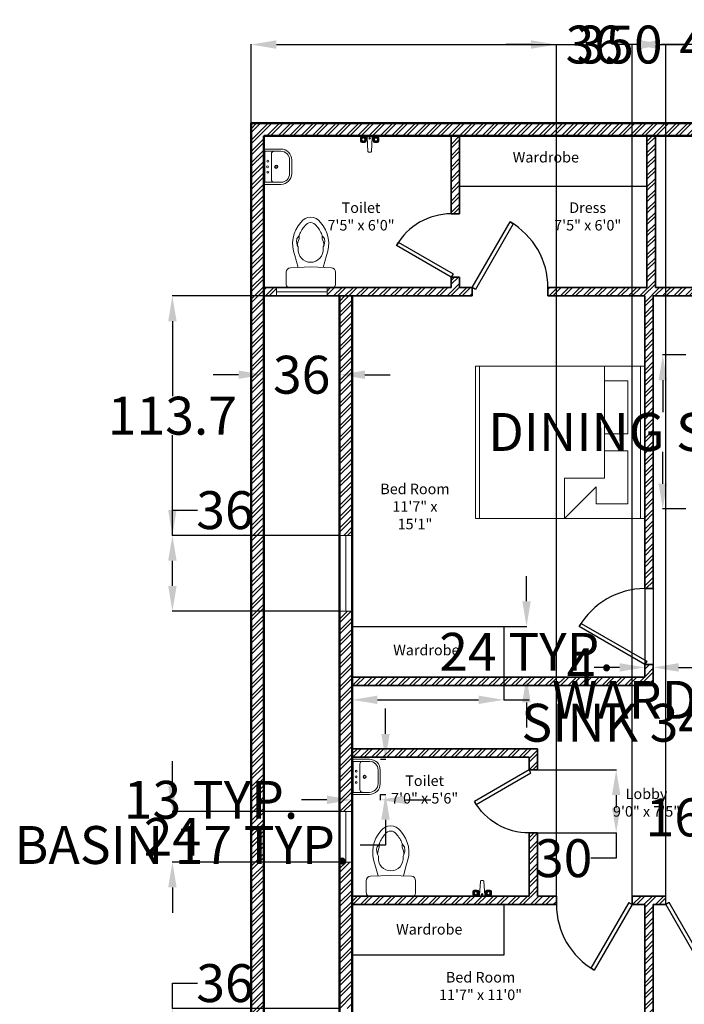
# Model space of a CAD drawing. Units: inches. Extents: x 73 to 1216, y -495 to 328.
# Tile 2 of 9: x 73 to 389, y -139 to 328. Entities that reach past the tile are written whole.
import ezdxf

# ---------------------------------------------------------------- set-up
doc = ezdxf.new("R2010")
doc.units = ezdxf.units.IN
for name, color, linetype, lineweight in [('A-ANNO-DIMS', 2, 'Continuous', 18), ('A-AREA-IDEN', 7, 'Continuous', 18), ('A-DOOR', 3, 'Continuous', 25), ('A-FLOR-CASE', 2, 'Continuous', 25), ('A-FLOR-FIXT', 9, 'Continuous', 18), ('A-GLAZ', 3, 'Continuous', 18), ('A-WALL-PATT', 8, 'Continuous', 13), ('Furniture', 2, 'Continuous', 18), ('Inner Walls', 5, 'Continuous', 35), ('Outer Walls', 1, 'Continuous', 50), ('Text-T18', 7, 'Continuous', 18)]:
    doc.layers.add(name, color=color, linetype=linetype, lineweight=lineweight)
doc.styles.get("Standard").update_dxf_attribs({"font": 'arial.ttf'})
doc.dimstyles.get("Standard").update_dxf_attribs({"dimtxt": 18, "dimasz": 12, "dimexe": 0.18, "dimexo": 0.0625, "dimgap": 0.09, "dimtad": 0, "dimtih": 1, "dimtoh": 1, "dimdec": 0, "dimzin": 0, "dimdsep": 46, "dimlunit": 3, "dimtxsty": 'Standard', "dimcen": 0.09, "dimadec": 0, "dimazin": 0, "dimtfac": 1, "dimtdec": 0, "dimtofl": 0, "dimtmove": 0, "dimatfit": 3, "dimfxl": 1, "dimtolj": 1, "dimtzin": 0, "dimarcsym": 0})
pattern_1 = [(45, (-434.707, -1257.0093), (-2.694077, 2.694077), []), (45, (-432.911, -1257.0093), (-2.694077, 2.694077), [])]

# ---------------------------------------------------------------- blocks, each defined once
blk = doc.blocks.new('*U2')
for p, q in [((0, 0), (0, -4)), ((36, 0), (36, -4))]:
    blk.add_line(p, q)
blk.add_lwpolyline([(0, 0), (18, 31.18), (19.52, 30.3), (1.52, -0.88)], close=True)
blk.add_arc((0, 0), 36, 0, 60)
blk = doc.blocks.new('*U3')
for p, q in [((0, 0), (0, -4)), ((30, 0), (30, -4))]:
    blk.add_line(p, q)
blk.add_lwpolyline([(0, 0), (15, 25.98), (16.52, 25.11), (1.52, -0.88)], close=True)
blk.add_arc((0, 0), 30, 0, 60)
blk = doc.blocks.new('*U4')
for p, q in [((0, 0), (0, -4)), ((40, 0), (40, -4))]:
    blk.add_line(p, q)
blk.add_lwpolyline([(0, 0), (20, 34.64), (21.52, 33.77), (1.52, -0.88)], close=True)
blk.add_arc((0, 0), 40, 0, 60)
blk = doc.blocks.new('KING-00')
for p, q in [((-0.897, -0.947), (-0.897, 0.882)), ((0.602, 0.882), (0.602, -0.464)), ((1.034, -0.947), (1.034, 0.882)), ((0.602, 0.704), (0.881, 0.704)), ((0.881, 0.069), (0.881, 0.704)), ((0.602, 0.069), (0.881, 0.069)), ((0.881, -0.134), (0.602, -0.134)), ((0.881, -0.769), (0.881, -0.134)), ((0.119, -0.464), (0.119, -0.947)), ((0.602, -0.464), (0.119, -0.464)), ((0.119, -0.947), (0.5, -0.566)), ((0.5, -0.769), (0.5, -0.566)), ((0.5, -0.769), (0.881, -0.769))]:
    blk.add_line(p, q)
blk.add_lwpolyline([(-0.948, -0.947), (-0.948, 0.882), (1.084, 0.882), (1.084, -0.947)], close=True)
blk = doc.blocks.new('A$C1308471B')
at = {"ltscale": 20}
for p, q in [((0.0354, 0.4793), (0.1495, 0.4793)), ((0, 0.4607), (0, 0.0186)), ((0.2013, 0.2397), (0.1923, 0.4384)), ((0.1957, 0.3639), (0.3109, 0.3953)), ((0.5021, 0.3528), (0.4724, 0.3528)), ((0.4982, 0.3575), (0.4822, 0.3709)), ((0.2013, 0.2397), (0.1923, 0.0409)), ((0.1959, 0.1193), (0.3109, 0.0879)), ((0.5021, 0.1304), (0.4724, 0.1304)), ((0.4982, 0.1257), (0.4822, 0.1123)), ((0.0354, 0), (0.1495, 0))]:
    blk.add_line(p, q, dxfattribs=at)
for centre, radius, start, end in [((0.0354, 0.4328), 0.0465, 90, 136.52689), ((0.1495, 0.4365), 0.0429, 2.57554, 90), ((0.006, 0.4607), 0.006, 136.52689, 180), ((0.4248, 0.1104), 0.3068, 47.41345, 111.79241), ((0.3654, 0.2416), 0.1206, 83.35226, 180), ((0.3823, 0.3868), 0.0255, 263.35226, 298.57415), ((0.4494, 0.2636), 0.1148, 79.39683, 118.57415), ((0.405, 0.2159), 0.153, 63.50202, 90.45216), ((0.4658, 0.3513), 0.0255, 50, 79.39683), ((0.5146, 0.377), 0.0255, 230, 251.38812), ((0.5021, 0.3273), 0.0255, 70.3751, 90), ((0.4248, 0.1104), 0.2558, 46.61198, 70.3751), ((0.5654, 0.2416), 0.065, 0, 57.29738), ((0.5654, 0.2416), 0.116, 0, 54.71147), ((0.3654, 0.2416), 0.1206, 180, 276.64774), ((0.5654, 0.2416), 0.065, 302.70262, 0), ((0.5654, 0.2416), 0.116, 305.28853, 0), ((0.4248, 0.3728), 0.3068, 248.20759, 312.58655), ((0.3823, 0.0964), 0.0255, 61.42585, 96.64774), ((0.4494, 0.2196), 0.1148, 241.42585, 280.60317), ((0.405, 0.2673), 0.153, 269.54784, 296.49798), ((0.4658, 0.1319), 0.0255, 280.60317, 310), ((0.5146, 0.1062), 0.0255, 108.61188, 130), ((0.5021, 0.1559), 0.0255, 270, 289.6249), ((0.4248, 0.3728), 0.2558, 289.6249, 313.38802), ((0.006, 0.0186), 0.006, 180, 223.47311), ((0.0354, 0.0465), 0.0465, 223.47311, 270), ((0.1495, 0.0429), 0.0429, 270, 357.42446)]:
    blk.add_arc(centre, radius, start, end, dxfattribs=at)
blk = doc.blocks.new('A$C57EA129C')
for p, q in [((0, 0.443), (0, 0.178)), ((0.016, 0.459), (0.563, 0.459)), ((0.036, 0.432), (0.036, 0.29)), ((0.045, 0.441), (0.535, 0.441)), ((0.08, 0.334), (0.499, 0.334)), ((0.544, 0.432), (0.544, 0.29)), ((0.579, 0.443), (0.579, 0.178)), ((0.036, 0.29), (0.036, 0.178)), ((0.544, 0.29), (0.544, 0.178)), ((0.178, 0.036), (0.401, 0.036)), ((0.178, 0), (0.401, 0))]:
    blk.add_line(p, q)
for centre, radius in [((0.198, 0.392), 0.0143), ((0.29, 0.396), 0.0156), ((0.381, 0.392), 0.0143), ((0.29, 0.255), 0.0267), ((0.29, 0.255), 0.0178)]:
    blk.add_circle(centre, radius)
for centre, radius, start, end in [((0.016, 0.443), 0.016, 90, 180), ((0.045, 0.432), 0.00891, 90, 180), ((0.08, 0.29), 0.0445, 90, 180), ((0.499, 0.29), 0.0445, 0, 90), ((0.535, 0.432), 0.00891, 0, 90), ((0.563, 0.443), 0.016, 0, 90), ((0.178, 0.178), 0.178, 180, 270), ((0.178, 0.178), 0.143, 180, 270), ((0.401, 0.178), 0.178, 270, 0), ((0.401, 0.178), 0.143, 270, 0)]:
    blk.add_arc(centre, radius, start, end)
blk = doc.blocks.new('A$C68D75330')
for p, q in [((0.155, 0.406), (0.155, 0.451)), ((0.167, 0.404), (0.167, 0.454)), ((0.172, 0.459), (0.222, 0.459)), ((0.175, 0.471), (0.22, 0.471)), ((0.227, 0.454), (0.227, 0.404)), ((0.24, 0.451), (0.24, 0.406)), ((0.264, 0.256), (0.252, 0.461)), ((0.275, 0.471), (0.305, 0.471)), ((0.327, 0.461), (0.315, 0.256)), ((0.34, 0.451), (0.34, 0.406)), ((0.352, 0.454), (0.352, 0.404)), ((0.407, 0.459), (0.357, 0.459)), ((0.405, 0.471), (0.36, 0.471)), ((0.412, 0.404), (0.412, 0.454)), ((0.425, 0.406), (0.425, 0.451)), ((0.222, 0.399), (0.172, 0.399)), ((0.22, 0.386), (0.175, 0.386)), ((0.357, 0.399), (0.407, 0.399)), ((0.36, 0.386), (0.405, 0.386)), ((0.306, 0.246), (0.274, 0.246))]:
    blk.add_line(p, q)
for centre, radius in [((0.197, 0.429), 0.03), ((0.197, 0.429), 0.0232), ((0.29, 0.446), 0.0125), ((0.29, 0.446), 0.00625), ((0.382, 0.429), 0.03), ((0.382, 0.429), 0.0232)]:
    blk.add_circle(centre, radius)
for centre, radius, start, end in [((0.175, 0.451), 0.02, 90, 180), ((0.172, 0.454), 0.005, 90, 180), ((0.22, 0.451), 0.02, 0, 90), ((0.222, 0.454), 0.005, 0, 90), ((0.274, 0.444), 0.0273, 87.1975, 140.7274), ((0.306, 0.444), 0.0273, 39.2726, 92.8025), ((0.36, 0.451), 0.02, 90, 180), ((0.357, 0.454), 0.005, 90, 180), ((0.405, 0.451), 0.02, 0, 90), ((0.407, 0.454), 0.005, 0, 90), ((0.175, 0.406), 0.02, 180, 270), ((0.172, 0.404), 0.005, 180, 270), ((0.22, 0.406), 0.02, 270, 0), ((0.222, 0.404), 0.005, 270, 0), ((0.36, 0.406), 0.02, 180, 270), ((0.357, 0.404), 0.005, 180, 270), ((0.405, 0.406), 0.02, 270, 0), ((0.407, 0.404), 0.005, 270, 0), ((0.274, 0.256), 0.01, 183.3274, 270), ((0.306, 0.256), 0.01, 270, 356.6726)]:
    blk.add_arc(centre, radius, start, end)
blk = doc.blocks.new('*U16')
for p, q in [((0, 6), (0, 0)), ((24, 6), (24, 0)), ((0, 3), (24, 3))]:
    blk.add_line(p, q)
blk = doc.blocks.new('*U17')
for p, q in [((0, 6), (0, 0)), ((36, 6), (36, 0)), ((0, 3), (36, 3))]:
    blk.add_line(p, q)
blk = doc.blocks.new('*U18')
for p, q in [((0, 4), (0, 0)), ((0, 2), (24, 2)), ((24, 4), (24, 0))]:
    blk.add_line(p, q)
blk = doc.blocks.new('WARDROBE-72X24')
blk.add_lwpolyline([(0, 24), (72, 24), (72, 0), (0, 0)], close=True)
blk = doc.blocks.new('WARDROBE-89X24')
blk.add_lwpolyline([(0, 24), (89, 24), (89, 0), (0, 0)], close=True)
blk = doc.blocks.new('*D32')
at = {"layer": 'A-ANNO-DIMS', "color": 0, "lineweight": -2, "transparency": 16777216}
for p, q in [((246.69, -10.79), (246.69, 1.21)), ((244.24, -22.79), (246.87, -22.79)), ((244.24, -39.57), (246.87, -39.57)), ((246.69, -51.57), (246.69, -63.57)), ((246.69, -63.57), (234.69, -63.57))]:
    blk.add_line(p, q, dxfattribs=at)
at = {"layer": 'A-ANNO-DIMS', "color": 0, "transparency": 16777216}
for points in [[(244.69, -10.79), (248.69, -10.79), (246.69, -22.79)], [(244.69, -51.57), (248.69, -51.57), (246.69, -39.57)]]:
    blk.add_solid(points, dxfattribs=at)
at = {"layer": 'Defpoints', "color": 0, "transparency": 16777216}
for p in [(244.17, -22.79), (244.17, -39.57), (246.69, -39.57)]:
    blk.add_point(p, dxfattribs=at)
at = {"layer": 'A-ANNO-DIMS', "color": 0, "transparency": 16777216, "insert": (149.97, -63.57), "char_height": 18, "attachment_point": 5}
blk.add_mtext('\\A1;BASIN 17 TYP.', dxfattribs=at)
blk = doc.blocks.new('*D33')
at = {"layer": 'A-ANNO-DIMS', "color": 0, "lineweight": -2, "transparency": 16777216}
for p, q in [((230.87, -39.64), (230.87, -42.27)), ((244.17, -39.64), (244.17, -42.27)), ((218.87, -42.09), (206.87, -42.09)), ((256.17, -42.09), (268.17, -42.09))]:
    blk.add_line(p, q, dxfattribs=at)
at = {"layer": 'A-ANNO-DIMS', "color": 0, "transparency": 16777216}
for points in [[(218.87, -40.09), (218.87, -44.09), (230.87, -42.09)], [(256.17, -40.09), (256.17, -44.09), (244.17, -42.09)]]:
    blk.add_solid(points, dxfattribs=at)
at = {"layer": 'Defpoints', "color": 0, "transparency": 16777216}
for p in [(230.87, -39.57), (244.17, -39.57), (230.87, -42.09)]:
    blk.add_point(p, dxfattribs=at)
at = {"layer": 'A-ANNO-DIMS', "color": 0, "transparency": 16777216, "insert": (163.82, -42.09), "char_height": 18, "attachment_point": 5}
blk.add_mtext('\\A1;13 TYP.', dxfattribs=at)
blk = doc.blocks.new('*D36')
at = {"layer": 'A-ANNO-DIMS', "color": 0, "lineweight": -2, "transparency": 16777216}
for p, q in [((230.87, 16.11), (230.87, 5.2)), ((302.87, 16.11), (302.87, 5.2)), ((242.87, 5.38), (290.87, 5.38)), ((302.87, 5.38), (314.87, 5.38))]:
    blk.add_line(p, q, dxfattribs=at)
at = {"layer": 'A-ANNO-DIMS', "color": 0, "transparency": 16777216}
for points in [[(242.87, 7.38), (242.87, 3.38), (230.87, 5.38)], [(290.87, 7.38), (290.87, 3.38), (302.87, 5.38)]]:
    blk.add_solid(points, dxfattribs=at)
at = {"layer": 'Defpoints', "color": 0, "transparency": 16777216}
for p in [(230.87, 16.18), (302.87, 16.18), (302.87, 5.38)]:
    blk.add_point(p, dxfattribs=at)
at = {"layer": 'A-ANNO-DIMS', "color": 0, "transparency": 16777216, "insert": (436.68, 5.38), "char_height": 18, "attachment_point": 5}
blk.add_mtext('\\A1;WARDROBE 72 TYP.', dxfattribs=at)
blk = doc.blocks.new('*D37')
at = {"layer": 'A-ANNO-DIMS', "color": 0, "lineweight": -2, "transparency": 16777216}
for p, q in [((313.67, 52.18), (313.67, 64.18)), ((302.94, 40.18), (313.85, 40.18)), ((302.94, 16.18), (313.85, 16.18)), ((313.67, 4.18), (313.67, -7.82))]:
    blk.add_line(p, q, dxfattribs=at)
at = {"layer": 'A-ANNO-DIMS', "color": 0, "transparency": 16777216}
for points in [[(311.67, 52.18), (315.67, 52.18), (313.67, 40.18)], [(311.67, 4.18), (315.67, 4.18), (313.67, 16.18)]]:
    blk.add_solid(points, dxfattribs=at)
at = {"layer": 'Defpoints', "color": 0, "transparency": 16777216}
for p in [(302.87, 40.18), (313.67, 40.18), (302.87, 16.18)]:
    blk.add_point(p, dxfattribs=at)
at = {"layer": 'A-ANNO-DIMS', "color": 0, "transparency": 16777216, "insert": (313.67, 28.18), "char_height": 18, "attachment_point": 5}
blk.add_mtext('\\A1;24 TYP.', dxfattribs=at)
blk = doc.blocks.new('*D44')
at = {"layer": 'A-ANNO-DIMS', "color": 0, "lineweight": -2, "transparency": 16777216}
for p, q in [((471.83, -5.5), (459.83, -5.5)), ((471.83, -10.54), (471.83, -5.32)), ((493.84, -5.5), (483.83, -5.5)), ((505.84, -10.54), (505.84, -5.32))]:
    blk.add_line(p, q, dxfattribs=at)
at = {"layer": 'A-ANNO-DIMS', "color": 0, "transparency": 16777216}
for points in [[(483.83, -3.5), (483.83, -7.5), (471.83, -5.5)], [(493.84, -3.5), (493.84, -7.5), (505.84, -5.5)]]:
    blk.add_solid(points, dxfattribs=at)
at = {"layer": 'Defpoints', "color": 0, "transparency": 16777216}
for p in [(471.83, -5.5), (471.83, -10.6), (505.84, -10.6)]:
    blk.add_point(p, dxfattribs=at)
at = {"layer": 'A-ANNO-DIMS', "color": 0, "transparency": 16777216, "insert": (383.14, -5.5), "char_height": 18, "attachment_point": 5}
blk.add_mtext('\\A1;SINK 34 TYP.', dxfattribs=at)
blk = doc.blocks.new('*D45')
at = {"layer": 'A-ANNO-DIMS', "color": 0, "lineweight": -2, "transparency": 16777216}
for p, q in [((466.73, 1.4), (466.73, 13.4)), ((471.77, -10.6), (466.55, -10.6)), ((471.77, -26.44), (466.55, -26.44)), ((466.73, -38.44), (466.73, -50.44)), ((466.73, -50.44), (454.73, -50.44))]:
    blk.add_line(p, q, dxfattribs=at)
at = {"layer": 'A-ANNO-DIMS', "color": 0, "transparency": 16777216}
for points in [[(464.73, 1.4), (468.73, 1.4), (466.73, -10.6)], [(464.73, -38.44), (468.73, -38.44), (466.73, -26.44)]]:
    blk.add_solid(points, dxfattribs=at)
at = {"layer": 'Defpoints', "color": 0, "transparency": 16777216}
for p in [(471.83, -10.6), (466.73, -26.44), (471.83, -26.44)]:
    blk.add_point(p, dxfattribs=at)
at = {"layer": 'A-ANNO-DIMS', "color": 0, "transparency": 16777216, "insert": (411.68, -50.44), "char_height": 18, "attachment_point": 5}
blk.add_mtext('\\A1;16 TYP.', dxfattribs=at)
blk = doc.blocks.new('*D48')
at = {"layer": 'A-ANNO-DIMS', "color": 0, "lineweight": -2, "transparency": 16777216}
for p, q in [((389.31, 169.17), (378.22, 169.17)), ((378.4, 157.17), (378.4, 141.99)), ((378.4, 108.01), (378.4, 123.19)), ((389.31, 96.01), (378.22, 96.01))]:
    blk.add_line(p, q, dxfattribs=at)
at = {"layer": 'A-ANNO-DIMS', "color": 0, "transparency": 16777216}
for points in [[(376.4, 157.17), (380.4, 157.17), (378.4, 169.17)], [(376.4, 108.01), (380.4, 108.01), (378.4, 96.01)]]:
    blk.add_solid(points, dxfattribs=at)
at = {"layer": 'Defpoints', "color": 0, "transparency": 16777216}
for p in [(389.37, 169.17), (378.4, 96.01), (389.37, 96.01)]:
    blk.add_point(p, dxfattribs=at)
at = {"layer": 'A-ANNO-DIMS', "color": 0, "transparency": 16777216, "insert": (378.4, 132.59), "char_height": 18, "attachment_point": 5}
blk.add_mtext('\\A1;DINING SET 73', dxfattribs=at)
blk = doc.blocks.new('*D50')
at = {"layer": 'A-ANNO-DIMS', "color": 0, "lineweight": -2, "transparency": 16777216}
for p, q in [((182.87, 279.24), (182.87, 316.76)), ((194.87, 316.58), (337.94, 316.58)), ((520.87, 316.58), (377.81, 316.58)), ((532.87, 279.24), (532.87, 316.76))]:
    blk.add_line(p, q, dxfattribs=at)
at = {"layer": 'A-ANNO-DIMS', "color": 0, "transparency": 16777216}
for points in [[(194.87, 318.58), (194.87, 314.58), (182.87, 316.58)], [(520.87, 318.58), (520.87, 314.58), (532.87, 316.58)]]:
    blk.add_solid(points, dxfattribs=at)
at = {"layer": 'Defpoints', "color": 0, "transparency": 16777216}
for p in [(532.87, 316.58), (182.87, 279.18), (532.87, 279.18)]:
    blk.add_point(p, dxfattribs=at)
at = {"layer": 'A-ANNO-DIMS', "color": 0, "transparency": 16777216, "insert": (357.87, 316.58), "char_height": 18, "attachment_point": 5}
blk.add_mtext('\\A1;350', dxfattribs=at)
blk = doc.blocks.new('*D54')
at = {"layer": 'A-ANNO-DIMS', "color": 0, "lineweight": -2, "transparency": 16777216}
for p, q in [((188.87461, 197.113801), (188.87461, 159.596301)), ((224.87461, 197.113801), (224.87461, 159.596301)), ((176.87461, 159.776301), (164.87461, 159.776301)), ((236.87461, 159.776301), (248.87461, 159.776301))]:
    blk.add_line(p, q, dxfattribs=at)
at = {"layer": 'A-ANNO-DIMS', "color": 0, "transparency": 16777216}
for points in [[(176.87461, 161.776301), (176.87461, 157.776301), (188.87461, 159.776301)], [(236.87461, 161.776301), (236.87461, 157.776301), (224.87461, 159.776301)]]:
    blk.add_solid(points, dxfattribs=at)
at = {"layer": 'Defpoints', "color": 0, "transparency": 16777216}
for p in [(188.87461, 197.176301), (224.87461, 197.176301), (188.87461, 159.776301)]:
    blk.add_point(p, dxfattribs=at)
at = {"layer": 'A-ANNO-DIMS', "color": 0, "transparency": 16777216, "insert": (206.87461, 159.776301), "char_height": 18, "attachment_point": 5}
blk.add_mtext('\\A1;36', dxfattribs=at)
blk = doc.blocks.new('*D61')
at = {"layer": 'A-ANNO-DIMS', "color": 0, "lineweight": -2, "transparency": 16777216}
for p, q in [((315.87461, 316.576301), (303.87461, 316.576301)), ((327.87461, -87.761199), (327.87461, 316.756301)), ((363.87461, -87.761199), (363.87461, 316.756301)), ((375.87461, 316.576301), (387.87461, 316.576301))]:
    blk.add_line(p, q, dxfattribs=at)
at = {"layer": 'A-ANNO-DIMS', "color": 0, "transparency": 16777216}
for points in [[(315.87461, 318.576301), (315.87461, 314.576301), (327.87461, 316.576301)], [(375.87461, 318.576301), (375.87461, 314.576301), (363.87461, 316.576301)]]:
    blk.add_solid(points, dxfattribs=at)
at = {"layer": 'Defpoints', "color": 0, "transparency": 16777216}
for p in [(363.87461, 316.576301), (327.87461, -87.823699), (363.87461, -87.823699)]:
    blk.add_point(p, dxfattribs=at)
at = {"layer": 'A-ANNO-DIMS', "color": 0, "transparency": 16777216, "insert": (345.87461, 316.576301), "char_height": 18, "attachment_point": 5}
blk.add_mtext('\\A1;36', dxfattribs=at)
blk = doc.blocks.new('*D62')
at = {"layer": 'A-ANNO-DIMS', "color": 0, "lineweight": -2, "transparency": 16777216}
for p, q in [((367.87461, 316.576301), (355.87461, 316.576301)), ((379.87461, -87.761199), (379.87461, 316.756301)), ((419.87461, -87.761199), (419.87461, 316.756301)), ((431.87461, 316.576301), (443.87461, 316.576301))]:
    blk.add_line(p, q, dxfattribs=at)
at = {"layer": 'A-ANNO-DIMS', "color": 0, "transparency": 16777216}
for points in [[(367.87461, 318.576301), (367.87461, 314.576301), (379.87461, 316.576301)], [(431.87461, 318.576301), (431.87461, 314.576301), (419.87461, 316.576301)]]:
    blk.add_solid(points, dxfattribs=at)
at = {"layer": 'Defpoints', "color": 0, "transparency": 16777216}
for p in [(419.87461, 316.576301), (379.87461, -87.823699), (419.87461, -87.823699)]:
    blk.add_point(p, dxfattribs=at)
at = {"layer": 'A-ANNO-DIMS', "color": 0, "transparency": 16777216, "insert": (399.87461, 316.576301), "char_height": 18, "attachment_point": 5}
blk.add_mtext('\\A1;40', dxfattribs=at)
blk = doc.blocks.new('*D63')
at = {"layer": 'A-ANNO-DIMS', "color": 0, "lineweight": -2, "transparency": 16777216}
for p, q in [((318.94, -27.82), (356.45, -27.82)), ((356.27, -39.82), (356.27, -45.82)), ((318.94, -57.82), (356.45, -57.82)), ((356.27, -57.82), (356.27, -69.82)), ((356.27, -69.82), (344.27, -69.82))]:
    blk.add_line(p, q, dxfattribs=at)
at = {"layer": 'A-ANNO-DIMS', "color": 0, "transparency": 16777216}
for points in [[(354.27, -39.82), (358.27, -39.82), (356.27, -27.82)], [(354.27, -45.82), (358.27, -45.82), (356.27, -57.82)]]:
    blk.add_solid(points, dxfattribs=at)
at = {"layer": 'Defpoints', "color": 0, "transparency": 16777216}
for p in [(318.87, -27.82), (318.87, -57.82), (356.27, -57.82)]:
    blk.add_point(p, dxfattribs=at)
at = {"layer": 'A-ANNO-DIMS', "color": 0, "transparency": 16777216, "insert": (331.33, -69.82), "char_height": 18, "attachment_point": 5}
blk.add_mtext('\\A1;30', dxfattribs=at)
blk = doc.blocks.new('*D64')
at = {"layer": 'A-ANNO-DIMS', "color": 0, "lineweight": -2, "transparency": 16777216}
for p, q in [((145.47, -141.15), (145.47, -129.15)), ((145.47, -129.15), (157.47, -129.15)), ((224.81, -141.15), (145.29, -141.15)), ((145.47, -165.15), (145.47, -153.15)), ((224.81, -177.15), (145.29, -177.15))]:
    blk.add_line(p, q, dxfattribs=at)
at = {"layer": 'A-ANNO-DIMS', "color": 0, "transparency": 16777216}
for points in [[(143.47, -153.15), (147.47, -153.15), (145.47, -141.15)], [(143.47, -165.15), (147.47, -165.15), (145.47, -177.15)]]:
    blk.add_solid(points, dxfattribs=at)
at = {"layer": 'Defpoints', "color": 0, "transparency": 16777216}
for p in [(145.47, -141.15), (224.87, -141.15), (224.87, -177.15)]:
    blk.add_point(p, dxfattribs=at)
at = {"layer": 'A-ANNO-DIMS', "color": 0, "transparency": 16777216, "insert": (170.44, -129.15), "char_height": 18, "attachment_point": 5}
blk.add_mtext('\\A1;36', dxfattribs=at)
blk = doc.blocks.new('*D71')
at = {"layer": 'A-ANNO-DIMS', "color": 0, "lineweight": -2, "transparency": 16777216}
for p, q in [((369.87, 58.11), (369.87, 20.6)), ((373.87, 58.11), (373.87, 20.6)), ((357.87, 20.78), (345.87, 20.78)), ((385.87, 20.78), (397.87, 20.78))]:
    blk.add_line(p, q, dxfattribs=at)
at = {"layer": 'A-ANNO-DIMS', "color": 0, "transparency": 16777216}
for points in [[(357.87, 22.78), (357.87, 18.78), (369.87, 20.78)], [(385.87, 22.78), (385.87, 18.78), (373.87, 20.78)]]:
    blk.add_solid(points, dxfattribs=at)
at = {"layer": 'Defpoints', "color": 0, "transparency": 16777216}
for p in [(369.87, 58.18), (373.87, 58.18), (369.87, 20.78)]:
    blk.add_point(p, dxfattribs=at)
at = {"layer": 'A-ANNO-DIMS', "color": 0, "transparency": 16777216, "insert": (339.56, 20.78), "char_height": 18, "attachment_point": 5}
blk.add_mtext('\\A1;4', dxfattribs=at)
blk = doc.blocks.new('*D72')
at = {"layer": 'A-ANNO-DIMS', "color": 0, "lineweight": -2, "transparency": 16777216}
for p, q in [((145.47461, -35.698476), (145.47461, -23.698476)), ((224.81211, -47.698476), (145.29461, -47.698476)), ((224.81211, -71.698476), (145.29461, -71.698476)), ((145.47461, -83.698476), (145.47461, -95.698476))]:
    blk.add_line(p, q, dxfattribs=at)
at = {"layer": 'A-ANNO-DIMS', "color": 0, "transparency": 16777216}
for points in [[(143.47461, -35.698476), (147.47461, -35.698476), (145.47461, -47.698476)], [(143.47461, -83.698476), (147.47461, -83.698476), (145.47461, -71.698476)]]:
    blk.add_solid(points, dxfattribs=at)
at = {"layer": 'Defpoints', "color": 0, "transparency": 16777216}
for p in [(145.47461, -47.698476), (224.87461, -47.698476), (224.87461, -71.698476)]:
    blk.add_point(p, dxfattribs=at)
at = {"layer": 'A-ANNO-DIMS', "color": 0, "transparency": 16777216, "insert": (145.47461, -59.698476), "char_height": 18, "attachment_point": 5}
blk.add_mtext('\\A1;24', dxfattribs=at)
blk = doc.blocks.new('*D73')
at = {"layer": 'A-ANNO-DIMS', "color": 0, "lineweight": -2, "transparency": 16777216}
for p, q in [((145.47, 83.47), (145.47, 95.47)), ((145.47, 95.47), (157.47, 95.47)), ((224.81, 83.47), (145.29, 83.47)), ((145.47, 59.47), (145.47, 71.47)), ((224.81, 47.47), (145.29, 47.47))]:
    blk.add_line(p, q, dxfattribs=at)
at = {"layer": 'A-ANNO-DIMS', "color": 0, "transparency": 16777216}
for points in [[(143.47, 71.47), (147.47, 71.47), (145.47, 83.47)], [(143.47, 59.47), (147.47, 59.47), (145.47, 47.47)]]:
    blk.add_solid(points, dxfattribs=at)
at = {"layer": 'Defpoints', "color": 0, "transparency": 16777216}
for p in [(145.47, 83.47), (224.87, 83.47), (224.87, 47.47)]:
    blk.add_point(p, dxfattribs=at)
at = {"layer": 'A-ANNO-DIMS', "color": 0, "transparency": 16777216, "insert": (170.44, 95.47), "char_height": 18, "attachment_point": 5}
blk.add_mtext('\\A1;36', dxfattribs=at)
blk = doc.blocks.new('*D74')
at = {"layer": 'A-ANNO-DIMS', "color": 0, "lineweight": -2, "transparency": 16777216}
for p, q in [((224.81, 197.18), (145.29, 197.18)), ((145.47, 185.18), (145.47, 149.61)), ((145.47, 95.47), (145.47, 131.04)), ((224.81, 83.47), (145.29, 83.47))]:
    blk.add_line(p, q, dxfattribs=at)
at = {"layer": 'A-ANNO-DIMS', "color": 0, "transparency": 16777216}
for points in [[(143.47, 185.18), (147.47, 185.18), (145.47, 197.18)], [(143.47, 95.47), (147.47, 95.47), (145.47, 83.47)]]:
    blk.add_solid(points, dxfattribs=at)
at = {"layer": 'Defpoints', "color": 0, "transparency": 16777216}
for p in [(145.47, 197.18), (224.87, 197.18), (224.87, 83.47)]:
    blk.add_point(p, dxfattribs=at)
at = {"layer": 'A-ANNO-DIMS', "color": 0, "transparency": 16777216, "insert": (145.47, 140.32), "char_height": 18, "attachment_point": 5}
blk.add_mtext('\\A1;113.7', dxfattribs=at)

msp = doc.modelspace()

# ---------------------------------------------------------------- hatches: boundary and pattern name
at = {"layer": 'A-WALL-PATT'}
h = msp.add_hatch(dxfattribs=at)
h.set_pattern_fill('ANSI32', color=256, scale=0.4)
h.set_pattern_definition(pattern_1)
h.paths.add_polyline_path([(526.8746, -307.8237), (365.8746, -307.8237), (365.8746, -421.8237), (369.8746, -421.8237), (369.8746, -313.8237), (526.8746, -313.8237)], flags=17)
h.paths.add_polyline_path([(532.8746, 279.1763), (182.8746, 279.1763), (182.8746, -427.8237), (235.8746, -427.8237), (235.8746, -421.8237), (188.8746, -421.8237), (188.8746, 273.1763), (526.8746, 273.1763), (526.8746, -421.8237), (355.8746, -421.8237), (355.8746, -427.8237), (532.8746, -427.8237)])
h.paths.add_polyline_path([(230.8746, 197.1763), (224.8746, 197.1763), (224.8746, 83.4706), (230.8746, 83.4706)], flags=17)
h = msp.add_hatch(dxfattribs=at)
h.set_pattern_fill('ANSI32', color=256, scale=0.4)
h.set_pattern_definition(pattern_1)
h.paths.add_polyline_path([(287.8746, 201.1763), (281.8746, 201.1763), (281.8746, 206.1763), (277.8746, 206.1763), (277.8746, 201.1763), (218.9775, 201.1763), (218.9775, 197.1763), (287.8746, 197.1763)])
h.paths.add_polyline_path([(194.9775, 201.1763), (188.8746, 201.1763), (188.8746, 197.1763), (194.9775, 197.1763)])
h.paths.add_polyline_path([(281.8746, 273.1763), (277.8746, 273.1763), (277.8746, 236.1763), (281.8746, 236.1763)])
h.paths.add_polyline_path([(420.8746, 201.1763), (374.8746, 201.1763), (374.8746, 273.1763), (370.8746, 273.1763), (370.8746, 249.1763), (370.8746, 201.1763), (323.8746, 201.1763), (323.8746, 197.1763), (369.8746, 197.1763), (369.8746, 58.1763), (373.8746, 58.1763), (373.8746, 197.1763), (420.8746, 197.1763)])
h.paths.add_polyline_path([(472.8746, 201.1763), (466.8746, 201.1763), (466.8746, 273.1763), (462.8746, 273.1763), (462.8746, 201.1763), (456.8746, 201.1763), (456.8746, 197.1763), (472.8746, 197.1763)])
h.paths.add_polyline_path([(526.8746, 201.1763), (502.8746, 201.1763), (502.8746, 197.1763), (526.8746, 197.1763)])
h.paths.add_polyline_path([(373.8746, 22.1763), (369.8746, 22.1763), (369.8746, 16.1763), (230.8746, 16.1763), (230.8746, 12.1763), (373.8746, 12.1763)])
h.paths.add_polyline_path([(318.8746, -17.8237), (230.8746, -17.8237), (230.8746, -21.8237), (314.8746, -21.8237), (314.8746, -27.8237), (318.8746, -27.8237)])
h.paths.add_polyline_path([(327.8746, -87.8237), (318.8746, -87.8237), (318.8746, -57.8237), (314.8746, -57.8237), (314.8746, -87.8237), (230.8746, -87.8237), (230.8746, -91.8237), (327.8746, -91.8237)])
h.paths.add_polyline_path([(379.8746, -87.8237), (363.8746, -87.8237), (363.8746, -91.8237), (369.8746, -91.8237), (369.8746, -223.8237), (373.8746, -223.8237), (373.8746, -91.8237), (379.8746, -91.8237)])
h.paths.add_polyline_path([(448.8746, -87.8237), (430.8746, -87.8237), (430.8746, -33.8237), (436.8746, -33.8237), (436.8746, -29.8237), (426.8746, -29.8237), (426.8746, -87.8237), (419.8746, -87.8237), (419.8746, -91.8237), (448.8746, -91.8237)])
h.paths.add_polyline_path([(526.8746, -87.8237), (508.8746, -87.8237), (508.8746, -91.8237), (526.8746, -91.8237)])
h.paths.add_polyline_path([(526.8746, -29.8237), (514.8746, -29.8237), (514.8746, -33.8237), (526.8746, -33.8237)])
h.paths.add_polyline_path([(478.8746, -29.8237), (466.8746, -29.8237), (466.8746, -33.8237), (478.8746, -33.8237)])
h = msp.add_hatch(dxfattribs=at)
h.set_pattern_fill('ANSI32', color=256, scale=0.4)
h.set_pattern_definition(pattern_1)
h.paths.add_polyline_path([(230.8746, -71.6985), (224.8746, -71.6985), (224.8746, -141.1467), (230.8746, -141.1467)])
h.paths.add_polyline_path([(230.8746, 47.4706), (224.8746, 47.4706), (224.8746, -47.6985), (230.8746, -47.6985)])
h.paths.add_polyline_path([(230.8746, -177.1467), (224.8746, -177.1467), (224.8746, -229.8237), (373.8746, -229.8237), (373.8746, -223.8237), (230.8746, -223.8237)])

# ---------------------------------------------------------------- linework, layer by layer
at = {"layer": 'Inner Walls'}
for p, q in [((277.8746, 273.1763), (277.8746, 236.1763)), ((281.8746, 273.1763), (281.8746, 236.1763)), ((370.8746, 273.1763), (370.8746, 201.1763)), ((374.8746, 273.1763), (374.8746, 201.1763)), ((277.8746, 236.1763), (281.8746, 236.1763)), ((277.8746, 206.1763), (277.8746, 201.1763)), ((281.8746, 206.1763), (277.8746, 206.1763)), ((281.8746, 206.1763), (281.8746, 201.1763)), ((277.8746, 201.1763), (188.8746, 201.1763)), ((287.8746, 201.1763), (281.8746, 201.1763)), ((287.8746, 201.1763), (287.8746, 197.1763)), ((370.8746, 201.1763), (323.8746, 201.1763)), ((323.8746, 197.1763), (323.8746, 201.1763)), ((420.8746, 201.1763), (374.8746, 201.1763)), ((287.8746, 197.1763), (188.8746, 197.1763)), ((369.8746, 197.1763), (323.8746, 197.1763)), ((369.8746, 197.1763), (369.8746, 58.1763)), ((373.8746, 197.1763), (373.8746, 58.1763)), ((420.8746, 197.1763), (373.8746, 197.1763)), ((373.8746, 58.1763), (369.8746, 58.1763)), ((373.8746, 22.1763), (369.8746, 22.1763)), ((369.8746, 22.1763), (369.8746, 16.1763)), ((373.8746, 22.1763), (373.8746, 12.1763)), ((369.8746, 16.1763), (230.8746, 16.1763)), ((373.8746, 12.1763), (230.8746, 12.1763)), ((318.8746, -17.8237), (230.8746, -17.8237)), ((318.8746, -27.8237), (318.8746, -17.8237)), ((314.8746, -21.8237), (230.8746, -21.8237)), ((314.8746, -27.8237), (314.8746, -21.8237)), ((314.8746, -27.8237), (318.8746, -27.8237)), ((314.8746, -87.8237), (314.8746, -57.8237)), ((318.8746, -57.8237), (314.8746, -57.8237)), ((318.8746, -87.8237), (318.8746, -57.8237)), ((314.8746, -87.8237), (230.8746, -87.8237)), ((327.8746, -87.8237), (318.8746, -87.8237)), ((327.8746, -91.8237), (327.8746, -87.8237)), ((363.8746, -91.8237), (363.8746, -87.8237)), ((363.8746, -87.8237), (379.8746, -87.8237)), ((327.8746, -91.8237), (230.8746, -91.8237)), ((369.8746, -91.8237), (363.8746, -91.8237)), ((369.8746, -223.8237), (369.8746, -91.8237)), ((373.8746, -223.8237), (373.8746, -91.8237)), ((373.8746, -91.8237), (379.8746, -91.8237))]:
    msp.add_line(p, q, dxfattribs=at)
at = {"layer": 'Outer Walls'}
for p, q in [((182.8746, -427.8237), (182.8746, 279.1763)), ((182.8746, 279.1763), (532.8746, 279.1763)), ((188.8746, 273.1763), (526.8746, 273.1763)), ((188.8746, -421.8237), (188.8746, 273.1763)), ((224.8746, -229.8237), (224.8746, 197.1763)), ((230.8746, -223.8237), (230.8746, 197.1763))]:
    msp.add_line(p, q, dxfattribs=at)

# ---------------------------------------------------------------- block references
at = {"layer": 'A-DOOR'}
for name, p, rotation in [('*U3', (277.8746, 206.1763), 90), ('*U2', (369.8746, 22.1763), 90), ('*U2', (363.8746, -91.8237), 180)]:
    msp.add_blockref(name, p, dxfattribs=dict(at, rotation=rotation))
msp.add_blockref('*U2', (287.8746, 201.1763), dxfattribs=at)
at = {"layer": 'A-DOOR', "xscale": -1}
for name, p, rotation in [('*U3', (314.8746, -27.8237), 90), ('*U4', (379.8746, -91.8237), 180)]:
    msp.add_blockref(name, p, dxfattribs=dict(at, rotation=rotation))
at = {"layer": 'A-FLOR-CASE'}
for name, p in [('WARDROBE-89X24', (281.875, 249.176)), ('WARDROBE-72X24', (230.875, 16.176)), ('WARDROBE-72X24', (230.875, -115.824))]:
    msp.add_blockref(name, p, dxfattribs=at)
at = {"layer": 'A-FLOR-FIXT', "xscale": 32.67217261962217, "yscale": 32.67217261962217, "zscale": 32.67217261962217}
msp.add_blockref('A$C68D75330', (229.6865, 257.4873), dxfattribs=at)
at = {"layer": 'A-FLOR-FIXT'}
for name, p, xscale, yscale, zscale, rotation in [('A$C57EA129C', (202.174, 266.948), -28.98333223671166, 28.98333223671166, 28.98333223671166, 90), ('A$C1308471B', (222.9711, 201.1763), 48.95497407897215, 48.95497407897215, 48.95497407897215, 89.99999999999996), ('A$C57EA129C', (244.174, -22.7892), -28.98333223671166, 28.98333223671166, 28.98333223671166, 90), ('A$C1308471B', (261.015, -87.8237), 48.95497407897215, 48.95497407897215, 48.95497407897215, 89.99999999999996), ('A$C68D75330', (302.0613, -72.4205), 32.67217261962217, 32.67217261962217, 32.67217261962217, 180)]:
    msp.add_blockref(name, p, dxfattribs=dict(at, xscale=xscale, yscale=yscale, zscale=zscale, rotation=rotation))
at = {"layer": 'A-GLAZ'}
msp.add_blockref('*U18', (194.9775, 197.1763), dxfattribs=at)
at = {"layer": 'A-GLAZ', "rotation": 270}
for name, p in [('*U17', (224.8746, 83.4706)), ('*U16', (224.8746, -47.6985))]:
    msp.add_blockref(name, p, dxfattribs=at)
at = {"layer": 'Furniture', "xscale": 39.60249106241186, "yscale": 39.60249106241186, "zscale": 39.60249106241186}
msp.add_blockref('KING-00', (326.9257, 128.9661), dxfattribs=at)

# ---------------------------------------------------------------- texts
at = {"layer": 'A-AREA-IDEN', "char_height": 5, "attachment_point": 3}
for s, width, insert in [('\\pxqc;{\\fTimes New Roman|b0|i0|c0|p18;Toilet\\P7\'5" x 6\'0"}', 37.203385, (253.6552, 241.6098)), ('\\pxqc;{\\fTimes New Roman|b0|i0|c0|p18;Dress\\P7\'5" x 6\'0"}', 37.203385, (361.3414, 241.6098)), ('\\pxqc;{\\fTimes New Roman|b0|i0|c0|p18;Bed Room\\P11\'7" x 15\'1"}', 37.203385, (279.2898, 108.0374)), ('\\pxqc;{\\fTimes New Roman|b0|i0|c0|p18;Toilet\\P7\'0" x 5\'6"}', 37.203385, (283.8813, -30.5277)), ('\\pxqc;{\\fTimes New Roman|b0|i0|c0|p18;Lobby\\P9\'0" x 7\'5"}', 49.101878, (395.2374, -36.7631)), ('\\pxqc;{\\fTimes New Roman|b0|i0|c0|p18;Bed Room \\P11\'7" x 11\'0"}', 49.101878, (316.392, -123.867))]:
    msp.add_mtext_dynamic_manual_height_columns(s, width=width, gutter_width=12.5, heights=[0], dxfattribs=dict(at, insert=insert))
at = {"layer": 'Text-T18', "char_height": 5, "attachment_point": 3}
for insert in [(347.4071, 265.5701), (290.6541, 31.5208), (292.0268, -101.0799)]:
    msp.add_mtext_dynamic_manual_height_columns('\\pxqc;{\\fTimes New Roman|b0|i0|c0|p18;Wardrobe}', width=49.101878, gutter_width=12.5, heights=[0], dxfattribs=dict(at, insert=insert))

# ---------------------------------------------------------------- dimensions: what is measured, and where the dimension line sits
at = {"layer": 'A-ANNO-DIMS'}
for base, p1, p2, picture, middle in [((532.8746, 316.5763), (182.8746, 279.1763), (532.8746, 279.1763), '*D50', (357.8746, 316.5763)), ((363.8746, 316.5763), (327.8746, -87.8237), (363.8746, -87.8237), '*D61', (345.8746, 316.5763)), ((419.8746, 316.5763), (379.8746, -87.8237), (419.8746, -87.8237), '*D62', (399.8746, 316.5763))]:
    dim = msp.add_linear_dim(base=base, p1=p1, p2=p2, dimstyle='Standard', override={"dimdec": 0, "dimlfac": 1, "dimrnd": 0, "dimzin": 0, "dimdsep": 46, "dimlunit": 2}, dxfattribs=at)
    dim.commit()
    dim.dimension.update_dxf_attribs({"geometry": picture, "text_midpoint": middle})
for base, p1, p2, angle, override, picture, middle in [((145.4746, 197.1763), (224.8746, 83.4706), (224.8746, 197.1763), 90, {"dimdec": 1, "dimlfac": 1, "dimrnd": 0, "dimzin": 0, "dimdsep": 46, "dimlunit": 2}, '*D74', (145.4746, 140.3234)), ((188.8746, 159.7763), (224.8746, 197.1763), (188.8746, 197.1763), 180, {"dimdec": 0, "dimlfac": 1, "dimrnd": 0, "dimzin": 0, "dimdsep": 46, "dimlunit": 2}, '*D54', (206.8746, 159.7763)), ((145.4746, 83.4706), (224.8746, 47.4706), (224.8746, 83.4706), 90, {"dimdec": 0, "dimlfac": 1, "dimrnd": 0, "dimzin": 0, "dimdsep": 46, "dimlunit": 2}, '*D73', (170.4446, 95.4706)), ((369.8746, 20.7763), (373.8746, 58.1763), (369.8746, 58.1763), 180, {"dimdec": 0, "dimlfac": 1, "dimrnd": 0, "dimzin": 0, "dimdsep": 46, "dimlunit": 2}, '*D71', (339.5595, 20.7763)), ((145.4746, -47.6985), (224.8746, -71.6985), (224.8746, -47.6985), 90, {"dimdec": 0, "dimlfac": 1, "dimrnd": 0, "dimzin": 0, "dimdsep": 46, "dimlunit": 2}, '*D72', (145.4746, -59.6985)), ((356.2746, -57.8237), (318.8746, -27.8237), (318.8746, -57.8237), 270, {"dimdec": 0, "dimlfac": 1, "dimrnd": 0, "dimzin": 0, "dimdsep": 46, "dimlunit": 2}, '*D63', (331.3292, -69.8237)), ((145.4746, -141.1467), (224.8746, -177.1467), (224.8746, -141.1467), 90, {"dimdec": 0, "dimlfac": 1, "dimrnd": 0, "dimzin": 0, "dimdsep": 46, "dimlunit": 2}, '*D64', (170.4446, -129.1467))]:
    dim = msp.add_linear_dim(base=base, p1=p1, p2=p2, angle=angle, dimstyle='Standard', override=override, dxfattribs=at)
    dim.commit()
    dim.dimension.update_dxf_attribs({"geometry": picture, "text_midpoint": middle})
for base, p1, p2, angle, text, picture, middle in [((378.3985, 96.0082), (389.3726, 169.169), (389.3726, 96.0082), 270, 'DINING SET <>', '*D48', (378.3985, 132.5886)), ((313.6746, 40.1763), (302.8746, 16.1763), (302.8746, 40.1763), 90, '<> TYP.', '*D37', (313.6746, 28.1763)), ((471.8322, -5.4987), (505.8405, -10.5999), (471.8322, -10.5999), 180, 'SINK <> TYP.', '*D44', (383.1378, -5.4987)), ((466.7309, -26.4423), (471.8322, -10.5999), (471.8322, -26.4423), 270, '<> TYP.', '*D45', (411.6791, -50.4423)), ((246.6919, -39.5749), (244.174, -22.7892), (244.174, -39.5749), 270, 'BASIN <> TYP.', '*D32', (149.9675, -63.5749)), ((230.8746, -42.0927), (244.174, -39.5749), (230.8746, -39.5749), 180, '<> TYP.', '*D33', (163.8228, -42.0927))]:
    dim = msp.add_linear_dim(base=base, p1=p1, p2=p2, angle=angle, text=text, dimstyle='Standard', override={"dimdec": 0, "dimlfac": 1, "dimrnd": 0, "dimzin": 0, "dimdsep": 46, "dimlunit": 2}, dxfattribs=at)
    dim.commit()
    dim.dimension.update_dxf_attribs({"geometry": picture, "text_midpoint": middle})
dim = msp.add_linear_dim(base=(302.8746, 5.3763), p1=(230.8746, 16.1763), p2=(302.8746, 16.1763), text='WARDROBE <> TYP.', dimstyle='Standard', override={"dimdec": 0, "dimlfac": 1, "dimrnd": 0, "dimzin": 0, "dimdsep": 46, "dimlunit": 2}, dxfattribs=at)
dim.commit()
dim.dimension.update_dxf_attribs({"geometry": '*D36', "text_midpoint": (436.6795, 5.3763)})

doc.saveas('drawing.dxf')
